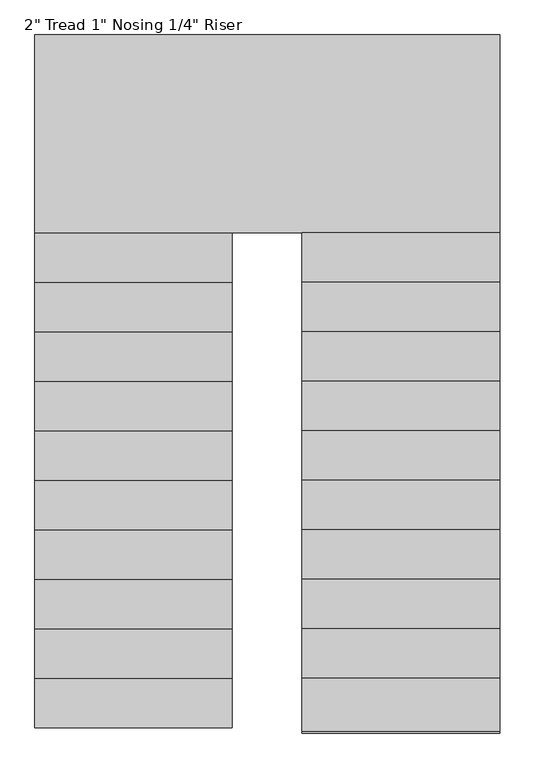
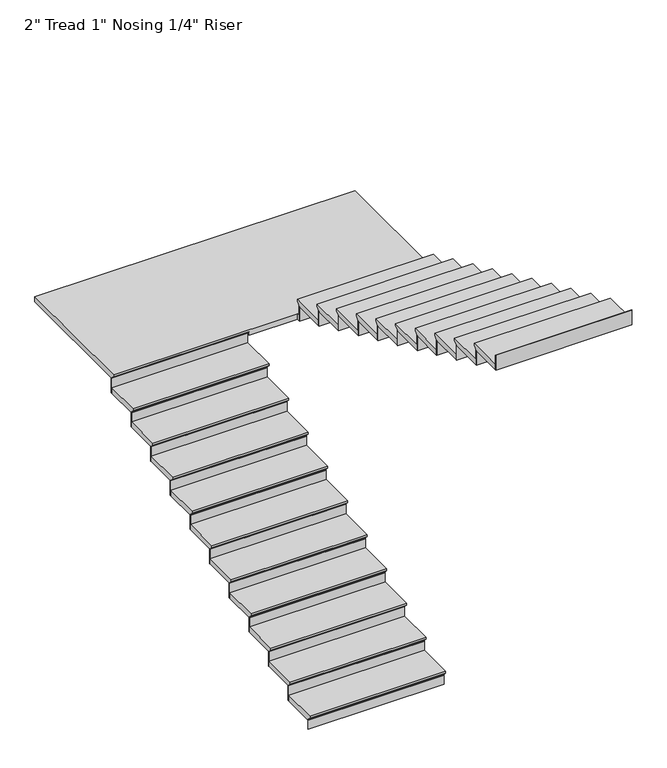
"""IFC4 building model written with IfcOpenShell, lengths in millimetres: stair flight geometry."""

from ifc_helpers import new_model, si_unit, origin, place, context, project, spatial, faceted_brep, source, transform, mapped, element, save


def stair_flight_f18b4829(model_context):
    return source(origin(), model_context, "Body", "Brep", [
        faceted_brep([(-629.5987998, 3364.6067329, 22522.2954545), (-629.5987998, 3364.6067329, 22541.3454545), (-1845.5417538, 3364.6067329, 22541.3454545), (-1845.5417538, 3364.6067329, 22522.2954545), (-629.5987998, 3390.0067329, 22496.8954545), (-1845.5417538, 3390.0067329, 22496.8954545), (-629.5987998, 3694.8067329, 22541.3454545), (-1845.5417538, 3694.8067329, 22541.3454545), (-1845.5417538, 3390.0067329, 22490.5454545), (-1845.5417538, 3694.8067329, 22490.5454545), (-629.5987998, 3694.8067329, 22490.5454545), (-629.5987998, 3390.0067329, 22490.5454545)], [[[0, 1, 2, 3]], [[4, 0, 3, 5]], [[2, 1, 6, 7]], [[8, 9, 10, 11]], [[2, 7, 9, 8, 5, 3]], [[8, 11, 4, 5]], [[6, 1, 0, 4, 11, 10]], [[7, 6, 10, 9]]]),
        faceted_brep([(-629.5987998, 3390.0067329, 22490.5454545), (-629.5987998, 3390.0067329, 22402.8), (-629.5987998, 3396.3567329, 22402.8), (-629.5987998, 3396.3567329, 22490.5454545), (-1845.5417538, 3390.0067329, 22490.5454545), (-1845.5417538, 3396.3567329, 22490.5454545), (-1845.5417538, 3396.3567329, 22402.8), (-1845.5417538, 3390.0067329, 22402.8)], [[[0, 1, 2, 3]], [[4, 5, 6, 7]], [[1, 0, 4, 7]], [[2, 1, 7, 6]], [[3, 2, 6, 5]], [[0, 3, 5, 4]]]),
        faceted_brep([(-629.5987998, 3694.8067329, 22629.0909091), (-629.5987998, 3694.8067329, 22490.5454545), (-629.5987998, 3701.1567329, 22490.5454545), (-629.5987998, 3701.1567329, 22629.0909091), (-1845.5417538, 3694.8067329, 22629.0909091), (-1845.5417538, 3701.1567329, 22629.0909091), (-1845.5417538, 3701.1567329, 22490.5454545), (-1845.5417538, 3694.8067329, 22490.5454545)], [[[0, 1, 2, 3]], [[4, 5, 6, 7]], [[1, 0, 4, 7]], [[2, 1, 7, 6]], [[3, 2, 6, 5]], [[0, 3, 5, 4]]]),
        faceted_brep([(-1845.5417538, 3669.4067329, 22679.8909091), (-629.5987998, 3669.4067329, 22679.8909091), (-629.5987998, 3999.6067329, 22679.8909091), (-1845.5417538, 3999.6067329, 22679.8909091), (-1845.5417538, 3694.8067329, 22629.0909091), (-1845.5417538, 3999.6067329, 22629.0909091), (-629.5987998, 3999.6067329, 22629.0909091), (-629.5987998, 3694.8067329, 22629.0909091), (-1845.5417538, 3694.8067329, 22635.4409091), (-1845.5417538, 3669.4067329, 22660.8409091), (-629.5987998, 3694.8067329, 22635.4409091), (-629.5987998, 3669.4067329, 22660.8409091)], [[[0, 1, 2, 3]], [[4, 5, 6, 7]], [[0, 3, 5, 4, 8, 9]], [[4, 7, 10, 8]], [[2, 1, 11, 10, 7, 6]], [[3, 2, 6, 5]], [[11, 1, 0, 9]], [[10, 11, 9, 8]]]),
        faceted_brep([(-629.5987998, 3999.6067329, 22767.6363636), (-629.5987998, 3999.6067329, 22629.0909091), (-629.5987998, 4005.9567329, 22629.0909091), (-629.5987998, 4005.9567329, 22767.6363636), (-1845.5417538, 3999.6067329, 22767.6363636), (-1845.5417538, 4005.9567329, 22767.6363636), (-1845.5417538, 4005.9567329, 22629.0909091), (-1845.5417538, 3999.6067329, 22629.0909091)], [[[0, 1, 2, 3]], [[4, 5, 6, 7]], [[1, 0, 4, 7]], [[2, 1, 7, 6]], [[3, 2, 6, 5]], [[0, 3, 5, 4]]]),
        faceted_brep([(-1845.5417538, 3974.2067329, 22818.4363636), (-629.5987998, 3974.2067329, 22818.4363636), (-629.5987998, 4304.4067329, 22818.4363636), (-1845.5417538, 4304.4067329, 22818.4363636), (-1845.5417538, 3999.6067329, 22767.6363636), (-1845.5417538, 4304.4067329, 22767.6363636), (-629.5987998, 4304.4067329, 22767.6363636), (-629.5987998, 3999.6067329, 22767.6363636), (-1845.5417538, 3999.6067329, 22773.9863636), (-1845.5417538, 3974.2067329, 22799.3863636), (-629.5987998, 3999.6067329, 22773.9863636), (-629.5987998, 3974.2067329, 22799.3863636)], [[[0, 1, 2, 3]], [[4, 5, 6, 7]], [[0, 3, 5, 4, 8, 9]], [[4, 7, 10, 8]], [[2, 1, 11, 10, 7, 6]], [[3, 2, 6, 5]], [[11, 1, 0, 9]], [[10, 11, 9, 8]]]),
        faceted_brep([(-629.5987998, 4304.4067329, 22906.1818182), (-629.5987998, 4304.4067329, 22767.6363636), (-629.5987998, 4310.7567329, 22767.6363636), (-629.5987998, 4310.7567329, 22906.1818182), (-1845.5417538, 4304.4067329, 22906.1818182), (-1845.5417538, 4310.7567329, 22906.1818182), (-1845.5417538, 4310.7567329, 22767.6363636), (-1845.5417538, 4304.4067329, 22767.6363636)], [[[0, 1, 2, 3]], [[4, 5, 6, 7]], [[1, 0, 4, 7]], [[2, 1, 7, 6]], [[3, 2, 6, 5]], [[0, 3, 5, 4]]]),
        faceted_brep([(-1845.5417538, 4279.0067329, 22956.9818182), (-629.5987998, 4279.0067329, 22956.9818182), (-629.5987998, 4609.2067329, 22956.9818182), (-1845.5417538, 4609.2067329, 22956.9818182), (-1845.5417538, 4304.4067329, 22906.1818182), (-1845.5417538, 4609.2067329, 22906.1818182), (-629.5987998, 4609.2067329, 22906.1818182), (-629.5987998, 4304.4067329, 22906.1818182), (-1845.5417538, 4304.4067329, 22912.5318182), (-1845.5417538, 4279.0067329, 22937.9318182), (-629.5987998, 4304.4067329, 22912.5318182), (-629.5987998, 4279.0067329, 22937.9318182)], [[[0, 1, 2, 3]], [[4, 5, 6, 7]], [[0, 3, 5, 4, 8, 9]], [[4, 7, 10, 8]], [[2, 1, 11, 10, 7, 6]], [[3, 2, 6, 5]], [[11, 1, 0, 9]], [[10, 11, 9, 8]]]),
        faceted_brep([(-629.5987998, 4609.2067329, 23044.7272727), (-629.5987998, 4609.2067329, 22906.1818182), (-629.5987998, 4615.5567329, 22906.1818182), (-629.5987998, 4615.5567329, 23044.7272727), (-1845.5417538, 4609.2067329, 23044.7272727), (-1845.5417538, 4615.5567329, 23044.7272727), (-1845.5417538, 4615.5567329, 22906.1818182), (-1845.5417538, 4609.2067329, 22906.1818182)], [[[0, 1, 2, 3]], [[4, 5, 6, 7]], [[1, 0, 4, 7]], [[2, 1, 7, 6]], [[3, 2, 6, 5]], [[0, 3, 5, 4]]]),
        faceted_brep([(-1845.5417538, 4583.8067329, 23095.5272727), (-629.5987998, 4583.8067329, 23095.5272727), (-629.5987998, 4914.0067329, 23095.5272727), (-1845.5417538, 4914.0067329, 23095.5272727), (-1845.5417538, 4609.2067329, 23044.7272727), (-1845.5417538, 4914.0067329, 23044.7272727), (-629.5987998, 4914.0067329, 23044.7272727), (-629.5987998, 4609.2067329, 23044.7272727), (-1845.5417538, 4609.2067329, 23051.0772727), (-1845.5417538, 4583.8067329, 23076.4772727), (-629.5987998, 4609.2067329, 23051.0772727), (-629.5987998, 4583.8067329, 23076.4772727)], [[[0, 1, 2, 3]], [[4, 5, 6, 7]], [[0, 3, 5, 4, 8, 9]], [[4, 7, 10, 8]], [[2, 1, 11, 10, 7, 6]], [[3, 2, 6, 5]], [[11, 1, 0, 9]], [[10, 11, 9, 8]]]),
        faceted_brep([(-629.5987998, 4914.0067329, 23183.2727273), (-629.5987998, 4914.0067329, 23044.7272727), (-629.5987998, 4920.3567329, 23044.7272727), (-629.5987998, 4920.3567329, 23183.2727273), (-1845.5417538, 4914.0067329, 23183.2727273), (-1845.5417538, 4920.3567329, 23183.2727273), (-1845.5417538, 4920.3567329, 23044.7272727), (-1845.5417538, 4914.0067329, 23044.7272727)], [[[0, 1, 2, 3]], [[4, 5, 6, 7]], [[1, 0, 4, 7]], [[2, 1, 7, 6]], [[3, 2, 6, 5]], [[0, 3, 5, 4]]]),
        faceted_brep([(-1845.5417538, 4888.6067329, 23234.0727273), (-629.5987998, 4888.6067329, 23234.0727273), (-629.5987998, 5218.8067329, 23234.0727273), (-1845.5417538, 5218.8067329, 23234.0727273), (-1845.5417538, 4914.0067329, 23183.2727273), (-1845.5417538, 5218.8067329, 23183.2727273), (-629.5987998, 5218.8067329, 23183.2727273), (-629.5987998, 4914.0067329, 23183.2727273), (-1845.5417538, 4914.0067329, 23189.6227273), (-1845.5417538, 4888.6067329, 23215.0227273), (-629.5987998, 4914.0067329, 23189.6227273), (-629.5987998, 4888.6067329, 23215.0227273)], [[[0, 1, 2, 3]], [[4, 5, 6, 7]], [[0, 3, 5, 4, 8, 9]], [[4, 7, 10, 8]], [[2, 1, 11, 10, 7, 6]], [[3, 2, 6, 5]], [[11, 1, 0, 9]], [[10, 11, 9, 8]]]),
        faceted_brep([(-629.5987998, 5218.8067329, 23321.8181818), (-629.5987998, 5218.8067329, 23183.2727273), (-629.5987998, 5225.1567329, 23183.2727273), (-629.5987998, 5225.1567329, 23321.8181818), (-1845.5417538, 5218.8067329, 23321.8181818), (-1845.5417538, 5225.1567329, 23321.8181818), (-1845.5417538, 5225.1567329, 23183.2727273), (-1845.5417538, 5218.8067329, 23183.2727273)], [[[0, 1, 2, 3]], [[4, 5, 6, 7]], [[1, 0, 4, 7]], [[2, 1, 7, 6]], [[3, 2, 6, 5]], [[0, 3, 5, 4]]]),
        faceted_brep([(-1845.5417538, 5193.4067329, 23372.6181818), (-629.5987998, 5193.4067329, 23372.6181818), (-629.5987998, 5523.6067329, 23372.6181818), (-1845.5417538, 5523.6067329, 23372.6181818), (-1845.5417538, 5218.8067329, 23321.8181818), (-1845.5417538, 5523.6067329, 23321.8181818), (-629.5987998, 5523.6067329, 23321.8181818), (-629.5987998, 5218.8067329, 23321.8181818), (-1845.5417538, 5218.8067329, 23328.1681818), (-1845.5417538, 5193.4067329, 23353.5681818), (-629.5987998, 5218.8067329, 23328.1681818), (-629.5987998, 5193.4067329, 23353.5681818)], [[[0, 1, 2, 3]], [[4, 5, 6, 7]], [[0, 3, 5, 4, 8, 9]], [[4, 7, 10, 8]], [[2, 1, 11, 10, 7, 6]], [[3, 2, 6, 5]], [[11, 1, 0, 9]], [[10, 11, 9, 8]]]),
        faceted_brep([(-629.5987998, 5523.6067329, 23460.3636364), (-629.5987998, 5523.6067329, 23321.8181818), (-629.5987998, 5529.9567329, 23321.8181818), (-629.5987998, 5529.9567329, 23460.3636364), (-1845.5417538, 5523.6067329, 23460.3636364), (-1845.5417538, 5529.9567329, 23460.3636364), (-1845.5417538, 5529.9567329, 23321.8181818), (-1845.5417538, 5523.6067329, 23321.8181818)], [[[0, 1, 2, 3]], [[4, 5, 6, 7]], [[1, 0, 4, 7]], [[2, 1, 7, 6]], [[3, 2, 6, 5]], [[0, 3, 5, 4]]]),
        faceted_brep([(-1845.5417538, 5498.2067329, 23511.1636364), (-629.5987998, 5498.2067329, 23511.1636364), (-629.5987998, 5828.4067329, 23511.1636364), (-1845.5417538, 5828.4067329, 23511.1636364), (-1845.5417538, 5523.6067329, 23460.3636364), (-1845.5417538, 5828.4067329, 23460.3636364), (-629.5987998, 5828.4067329, 23460.3636364), (-629.5987998, 5523.6067329, 23460.3636364), (-1845.5417538, 5523.6067329, 23466.7136364), (-1845.5417538, 5498.2067329, 23492.1136364), (-629.5987998, 5523.6067329, 23466.7136364), (-629.5987998, 5498.2067329, 23492.1136364)], [[[0, 1, 2, 3]], [[4, 5, 6, 7]], [[0, 3, 5, 4, 8, 9]], [[4, 7, 10, 8]], [[2, 1, 11, 10, 7, 6]], [[3, 2, 6, 5]], [[11, 1, 0, 9]], [[10, 11, 9, 8]]]),
        faceted_brep([(-629.5987998, 5828.4067329, 23598.9090909), (-629.5987998, 5828.4067329, 23460.3636364), (-629.5987998, 5834.7567329, 23460.3636364), (-629.5987998, 5834.7567329, 23598.9090909), (-1845.5417538, 5828.4067329, 23598.9090909), (-1845.5417538, 5834.7567329, 23598.9090909), (-1845.5417538, 5834.7567329, 23460.3636364), (-1845.5417538, 5828.4067329, 23460.3636364)], [[[0, 1, 2, 3]], [[4, 5, 6, 7]], [[1, 0, 4, 7]], [[2, 1, 7, 6]], [[3, 2, 6, 5]], [[0, 3, 5, 4]]]),
        faceted_brep([(-1845.5417538, 5803.0067329, 23649.7090909), (-629.5987998, 5803.0067329, 23649.7090909), (-629.5987998, 6133.2067329, 23649.7090909), (-1845.5417538, 6133.2067329, 23649.7090909), (-1845.5417538, 5828.4067329, 23598.9090909), (-1845.5417538, 6133.2067329, 23598.9090909), (-629.5987998, 6133.2067329, 23598.9090909), (-629.5987998, 5828.4067329, 23598.9090909), (-1845.5417538, 5828.4067329, 23605.2590909), (-1845.5417538, 5803.0067329, 23630.6590909), (-629.5987998, 5828.4067329, 23605.2590909), (-629.5987998, 5803.0067329, 23630.6590909)], [[[0, 1, 2, 3]], [[4, 5, 6, 7]], [[0, 3, 5, 4, 8, 9]], [[4, 7, 10, 8]], [[2, 1, 11, 10, 7, 6]], [[3, 2, 6, 5]], [[11, 1, 0, 9]], [[10, 11, 9, 8]]]),
        faceted_brep([(-629.5987998, 6133.2067329, 23737.4545455), (-629.5987998, 6133.2067329, 23598.9090909), (-629.5987998, 6139.5567329, 23598.9090909), (-629.5987998, 6139.5567329, 23737.4545455), (-1845.5417538, 6133.2067329, 23737.4545455), (-1845.5417538, 6139.5567329, 23737.4545455), (-1845.5417538, 6139.5567329, 23598.9090909), (-1845.5417538, 6133.2067329, 23598.9090909)], [[[0, 1, 2, 3]], [[4, 5, 6, 7]], [[1, 0, 4, 7]], [[2, 1, 7, 6]], [[3, 2, 6, 5]], [[0, 3, 5, 4]]]),
        faceted_brep([(-1845.5417538, 6107.8067329, 23788.2545455), (-629.5987998, 6107.8067329, 23788.2545455), (-629.5987998, 6438.0067329, 23788.2545455), (-1845.5417538, 6438.0067329, 23788.2545455), (-1845.5417538, 6133.2067329, 23737.4545455), (-1845.5417538, 6438.0067329, 23737.4545455), (-629.5987998, 6438.0067329, 23737.4545455), (-629.5987998, 6133.2067329, 23737.4545455), (-1845.5417538, 6133.2067329, 23743.8045455), (-1845.5417538, 6107.8067329, 23769.2045455), (-629.5987998, 6133.2067329, 23743.8045455), (-629.5987998, 6107.8067329, 23769.2045455)], [[[0, 1, 2, 3]], [[4, 5, 6, 7]], [[0, 3, 5, 4, 8, 9]], [[4, 7, 10, 8]], [[2, 1, 11, 10, 7, 6]], [[3, 2, 6, 5]], [[11, 1, 0, 9]], [[10, 11, 9, 8]]]),
        faceted_brep([(-629.5987998, 6438.0067329, 23876.0), (-629.5987998, 6438.0067329, 23737.4545455), (-629.5987998, 6444.3567329, 23737.4545455), (-629.5987998, 6444.3567329, 23876.0), (-1845.5417538, 6438.0067329, 23876.0), (-1845.5417538, 6444.3567329, 23876.0), (-1845.5417538, 6444.3567329, 23737.4545455), (-1845.5417538, 6438.0067329, 23737.4545455)], [[[0, 1, 2, 3]], [[4, 5, 6, 7]], [[1, 0, 4, 7]], [[2, 1, 7, 6]], [[3, 2, 6, 5]], [[0, 3, 5, 4]]]),
        faceted_brep([(1021.4012085, 6387.2067329, 23926.8), (1021.4012085, 7631.8067329, 23926.8), (-1845.5417538, 7631.8067329, 23926.8), (-1845.5417538, 6412.6067329, 23926.8), (-197.7987915, 6412.6067329, 23926.8), (-197.7987915, 6387.2067329, 23926.8), (1021.4012085, 7631.8067329, 23876.0), (1021.4012085, 6387.2067329, 23876.0), (-197.7987915, 6387.2067329, 23876.0), (-197.7987915, 6412.6067329, 23876.0), (-629.5987998, 6412.6067329, 23876.0), (-629.5987998, 6438.0067329, 23876.0), (-1845.5417538, 6438.0067329, 23876.0), (-1845.5417538, 7631.8067329, 23876.0), (-629.5987998, 6438.0067329, 23882.35), (-1845.5417538, 6438.0067329, 23882.35), (-1845.5417538, 6412.6067329, 23907.75), (-629.5987998, 6412.6067329, 23907.75)], [[[0, 1, 2, 3, 4, 5]], [[6, 7, 8, 9, 10, 11, 12, 13]], [[1, 0, 7, 6]], [[2, 1, 6, 13]], [[12, 11, 14, 15]], [[4, 3, 16, 17, 10, 9]], [[5, 4, 9, 8]], [[0, 5, 8, 7]], [[16, 15, 14, 17]], [[3, 2, 13, 12, 15, 16]], [[11, 10, 17, 14]]]),
        faceted_brep([(-197.7987915, 6387.2067329, 24014.5454545), (-197.7987915, 6387.2067329, 23876.0), (-197.7987915, 6380.8567329, 23876.0), (-197.7987915, 6380.8567329, 24014.5454545), (1021.4012085, 6387.2067329, 24014.5454545), (1021.4012085, 6380.8567329, 24014.5454545), (1021.4012085, 6380.8567329, 23876.0), (1021.4012085, 6387.2067329, 23876.0)], [[[0, 1, 2, 3]], [[4, 5, 6, 7]], [[1, 0, 4, 7]], [[2, 1, 7, 6]], [[3, 2, 6, 5]], [[0, 3, 5, 4]]]),
        faceted_brep([(1021.4012085, 6412.6067329, 24065.3454545), (-197.7987915, 6412.6067329, 24065.3454545), (-197.7987915, 6082.4067329, 24065.3454545), (1021.4012085, 6082.4067329, 24065.3454545), (1021.4012085, 6387.2067329, 24014.5454545), (1021.4012085, 6082.4067329, 24014.5454545), (-197.7987915, 6082.4067329, 24014.5454545), (-197.7987915, 6387.2067329, 24014.5454545), (1021.4012085, 6387.2067329, 24020.8954545), (1021.4012085, 6412.6067329, 24046.2954545), (-197.7987915, 6387.2067329, 24020.8954545), (-197.7987915, 6412.6067329, 24046.2954545)], [[[0, 1, 2, 3]], [[4, 5, 6, 7]], [[0, 3, 5, 4, 8, 9]], [[4, 7, 10, 8]], [[2, 1, 11, 10, 7, 6]], [[3, 2, 6, 5]], [[11, 1, 0, 9]], [[10, 11, 9, 8]]]),
        faceted_brep([(-197.7987915, 6082.4067329, 24153.0909091), (-197.7987915, 6082.4067329, 24014.5454545), (-197.7987915, 6076.0567329, 24014.5454545), (-197.7987915, 6076.0567329, 24153.0909091), (1021.4012085, 6082.4067329, 24153.0909091), (1021.4012085, 6076.0567329, 24153.0909091), (1021.4012085, 6076.0567329, 24014.5454545), (1021.4012085, 6082.4067329, 24014.5454545)], [[[0, 1, 2, 3]], [[4, 5, 6, 7]], [[1, 0, 4, 7]], [[2, 1, 7, 6]], [[3, 2, 6, 5]], [[0, 3, 5, 4]]]),
        faceted_brep([(1021.4012085, 6107.8067329, 24203.8909091), (-197.7987915, 6107.8067329, 24203.8909091), (-197.7987915, 5777.6067329, 24203.8909091), (1021.4012085, 5777.6067329, 24203.8909091), (1021.4012085, 6082.4067329, 24153.0909091), (1021.4012085, 5777.6067329, 24153.0909091), (-197.7987915, 5777.6067329, 24153.0909091), (-197.7987915, 6082.4067329, 24153.0909091), (1021.4012085, 6082.4067329, 24159.4409091), (1021.4012085, 6107.8067329, 24184.8409091), (-197.7987915, 6082.4067329, 24159.4409091), (-197.7987915, 6107.8067329, 24184.8409091)], [[[0, 1, 2, 3]], [[4, 5, 6, 7]], [[0, 3, 5, 4, 8, 9]], [[4, 7, 10, 8]], [[2, 1, 11, 10, 7, 6]], [[3, 2, 6, 5]], [[11, 1, 0, 9]], [[10, 11, 9, 8]]]),
        faceted_brep([(-197.7987915, 5777.6067329, 24291.6363636), (-197.7987915, 5777.6067329, 24153.0909091), (-197.7987915, 5771.2567329, 24153.0909091), (-197.7987915, 5771.2567329, 24291.6363636), (1021.4012085, 5777.6067329, 24291.6363636), (1021.4012085, 5771.2567329, 24291.6363636), (1021.4012085, 5771.2567329, 24153.0909091), (1021.4012085, 5777.6067329, 24153.0909091)], [[[0, 1, 2, 3]], [[4, 5, 6, 7]], [[1, 0, 4, 7]], [[2, 1, 7, 6]], [[3, 2, 6, 5]], [[0, 3, 5, 4]]]),
        faceted_brep([(1021.4012085, 5803.0067329, 24342.4363636), (-197.7987915, 5803.0067329, 24342.4363636), (-197.7987915, 5472.8067329, 24342.4363636), (1021.4012085, 5472.8067329, 24342.4363636), (1021.4012085, 5777.6067329, 24291.6363636), (1021.4012085, 5472.8067329, 24291.6363636), (-197.7987915, 5472.8067329, 24291.6363636), (-197.7987915, 5777.6067329, 24291.6363636), (1021.4012085, 5777.6067329, 24297.9863636), (1021.4012085, 5803.0067329, 24323.3863636), (-197.7987915, 5777.6067329, 24297.9863636), (-197.7987915, 5803.0067329, 24323.3863636)], [[[0, 1, 2, 3]], [[4, 5, 6, 7]], [[0, 3, 5, 4, 8, 9]], [[4, 7, 10, 8]], [[2, 1, 11, 10, 7, 6]], [[3, 2, 6, 5]], [[11, 1, 0, 9]], [[10, 11, 9, 8]]]),
        faceted_brep([(-197.7987915, 5472.8067329, 24430.1818182), (-197.7987915, 5472.8067329, 24291.6363636), (-197.7987915, 5466.4567329, 24291.6363636), (-197.7987915, 5466.4567329, 24430.1818182), (1021.4012085, 5472.8067329, 24430.1818182), (1021.4012085, 5466.4567329, 24430.1818182), (1021.4012085, 5466.4567329, 24291.6363636), (1021.4012085, 5472.8067329, 24291.6363636)], [[[0, 1, 2, 3]], [[4, 5, 6, 7]], [[1, 0, 4, 7]], [[2, 1, 7, 6]], [[3, 2, 6, 5]], [[0, 3, 5, 4]]]),
        faceted_brep([(1021.4012085, 5498.2067329, 24480.9818182), (-197.7987915, 5498.2067329, 24480.9818182), (-197.7987915, 5168.0067329, 24480.9818182), (1021.4012085, 5168.0067329, 24480.9818182), (1021.4012085, 5472.8067329, 24430.1818182), (1021.4012085, 5168.0067329, 24430.1818182), (-197.7987915, 5168.0067329, 24430.1818182), (-197.7987915, 5472.8067329, 24430.1818182), (1021.4012085, 5472.8067329, 24436.5318182), (1021.4012085, 5498.2067329, 24461.9318182), (-197.7987915, 5472.8067329, 24436.5318182), (-197.7987915, 5498.2067329, 24461.9318182)], [[[0, 1, 2, 3]], [[4, 5, 6, 7]], [[0, 3, 5, 4, 8, 9]], [[4, 7, 10, 8]], [[2, 1, 11, 10, 7, 6]], [[3, 2, 6, 5]], [[11, 1, 0, 9]], [[10, 11, 9, 8]]]),
        faceted_brep([(-197.7987915, 5168.0067329, 24568.7272727), (-197.7987915, 5168.0067329, 24430.1818182), (-197.7987915, 5161.6567329, 24430.1818182), (-197.7987915, 5161.6567329, 24568.7272727), (1021.4012085, 5168.0067329, 24568.7272727), (1021.4012085, 5161.6567329, 24568.7272727), (1021.4012085, 5161.6567329, 24430.1818182), (1021.4012085, 5168.0067329, 24430.1818182)], [[[0, 1, 2, 3]], [[4, 5, 6, 7]], [[1, 0, 4, 7]], [[2, 1, 7, 6]], [[3, 2, 6, 5]], [[0, 3, 5, 4]]]),
        faceted_brep([(1021.4012085, 5193.4067329, 24619.5272727), (-197.7987915, 5193.4067329, 24619.5272727), (-197.7987915, 4863.2067329, 24619.5272727), (1021.4012085, 4863.2067329, 24619.5272727), (1021.4012085, 5168.0067329, 24568.7272727), (1021.4012085, 4863.2067329, 24568.7272727), (-197.7987915, 4863.2067329, 24568.7272727), (-197.7987915, 5168.0067329, 24568.7272727), (1021.4012085, 5168.0067329, 24575.0772727), (1021.4012085, 5193.4067329, 24600.4772727), (-197.7987915, 5168.0067329, 24575.0772727), (-197.7987915, 5193.4067329, 24600.4772727)], [[[0, 1, 2, 3]], [[4, 5, 6, 7]], [[0, 3, 5, 4, 8, 9]], [[4, 7, 10, 8]], [[2, 1, 11, 10, 7, 6]], [[3, 2, 6, 5]], [[11, 1, 0, 9]], [[10, 11, 9, 8]]]),
        faceted_brep([(-197.7987915, 4863.2067329, 24707.2727273), (-197.7987915, 4863.2067329, 24568.7272727), (-197.7987915, 4856.8567329, 24568.7272727), (-197.7987915, 4856.8567329, 24707.2727273), (1021.4012085, 4863.2067329, 24707.2727273), (1021.4012085, 4856.8567329, 24707.2727273), (1021.4012085, 4856.8567329, 24568.7272727), (1021.4012085, 4863.2067329, 24568.7272727)], [[[0, 1, 2, 3]], [[4, 5, 6, 7]], [[1, 0, 4, 7]], [[2, 1, 7, 6]], [[3, 2, 6, 5]], [[0, 3, 5, 4]]]),
        faceted_brep([(1021.4012085, 4888.6067329, 24758.0727273), (-197.7987915, 4888.6067329, 24758.0727273), (-197.7987915, 4558.4067329, 24758.0727273), (1021.4012085, 4558.4067329, 24758.0727273), (1021.4012085, 4863.2067329, 24707.2727273), (1021.4012085, 4558.4067329, 24707.2727273), (-197.7987915, 4558.4067329, 24707.2727273), (-197.7987915, 4863.2067329, 24707.2727273), (1021.4012085, 4863.2067329, 24713.6227273), (1021.4012085, 4888.6067329, 24739.0227273), (-197.7987915, 4863.2067329, 24713.6227273), (-197.7987915, 4888.6067329, 24739.0227273)], [[[0, 1, 2, 3]], [[4, 5, 6, 7]], [[0, 3, 5, 4, 8, 9]], [[4, 7, 10, 8]], [[2, 1, 11, 10, 7, 6]], [[3, 2, 6, 5]], [[11, 1, 0, 9]], [[10, 11, 9, 8]]]),
        faceted_brep([(-197.7987915, 4558.4067329, 24845.8181818), (-197.7987915, 4558.4067329, 24707.2727273), (-197.7987915, 4552.0567329, 24707.2727273), (-197.7987915, 4552.0567329, 24845.8181818), (1021.4012085, 4558.4067329, 24845.8181818), (1021.4012085, 4552.0567329, 24845.8181818), (1021.4012085, 4552.0567329, 24707.2727273), (1021.4012085, 4558.4067329, 24707.2727273)], [[[0, 1, 2, 3]], [[4, 5, 6, 7]], [[1, 0, 4, 7]], [[2, 1, 7, 6]], [[3, 2, 6, 5]], [[0, 3, 5, 4]]]),
        faceted_brep([(1021.4012085, 4583.8067329, 24896.6181818), (-197.7987915, 4583.8067329, 24896.6181818), (-197.7987915, 4253.6067329, 24896.6181818), (1021.4012085, 4253.6067329, 24896.6181818), (1021.4012085, 4558.4067329, 24845.8181818), (1021.4012085, 4253.6067329, 24845.8181818), (-197.7987915, 4253.6067329, 24845.8181818), (-197.7987915, 4558.4067329, 24845.8181818), (1021.4012085, 4558.4067329, 24852.1681818), (1021.4012085, 4583.8067329, 24877.5681818), (-197.7987915, 4558.4067329, 24852.1681818), (-197.7987915, 4583.8067329, 24877.5681818)], [[[0, 1, 2, 3]], [[4, 5, 6, 7]], [[0, 3, 5, 4, 8, 9]], [[4, 7, 10, 8]], [[2, 1, 11, 10, 7, 6]], [[3, 2, 6, 5]], [[11, 1, 0, 9]], [[10, 11, 9, 8]]]),
        faceted_brep([(-197.7987915, 4253.6067329, 24984.3636364), (-197.7987915, 4253.6067329, 24845.8181818), (-197.7987915, 4247.2567329, 24845.8181818), (-197.7987915, 4247.2567329, 24984.3636364), (1021.4012085, 4253.6067329, 24984.3636364), (1021.4012085, 4247.2567329, 24984.3636364), (1021.4012085, 4247.2567329, 24845.8181818), (1021.4012085, 4253.6067329, 24845.8181818)], [[[0, 1, 2, 3]], [[4, 5, 6, 7]], [[1, 0, 4, 7]], [[2, 1, 7, 6]], [[3, 2, 6, 5]], [[0, 3, 5, 4]]]),
        faceted_brep([(1021.4012085, 4279.0067329, 25035.1636364), (-197.7987915, 4279.0067329, 25035.1636364), (-197.7987915, 3948.8067329, 25035.1636364), (1021.4012085, 3948.8067329, 25035.1636364), (1021.4012085, 4253.6067329, 24984.3636364), (1021.4012085, 3948.8067329, 24984.3636364), (-197.7987915, 3948.8067329, 24984.3636364), (-197.7987915, 4253.6067329, 24984.3636364), (1021.4012085, 4253.6067329, 24990.7136364), (1021.4012085, 4279.0067329, 25016.1136364), (-197.7987915, 4253.6067329, 24990.7136364), (-197.7987915, 4279.0067329, 25016.1136364)], [[[0, 1, 2, 3]], [[4, 5, 6, 7]], [[0, 3, 5, 4, 8, 9]], [[4, 7, 10, 8]], [[2, 1, 11, 10, 7, 6]], [[3, 2, 6, 5]], [[11, 1, 0, 9]], [[10, 11, 9, 8]]]),
        faceted_brep([(-197.7987915, 3948.8067329, 25122.9090909), (-197.7987915, 3948.8067329, 24984.3636364), (-197.7987915, 3942.4567329, 24984.3636364), (-197.7987915, 3942.4567329, 25122.9090909), (1021.4012085, 3948.8067329, 25122.9090909), (1021.4012085, 3942.4567329, 25122.9090909), (1021.4012085, 3942.4567329, 24984.3636364), (1021.4012085, 3948.8067329, 24984.3636364)], [[[0, 1, 2, 3]], [[4, 5, 6, 7]], [[1, 0, 4, 7]], [[2, 1, 7, 6]], [[3, 2, 6, 5]], [[0, 3, 5, 4]]]),
        faceted_brep([(1021.4012085, 3974.2067329, 25173.7090909), (-197.7987915, 3974.2067329, 25173.7090909), (-197.7987915, 3644.0067329, 25173.7090909), (1021.4012085, 3644.0067329, 25173.7090909), (1021.4012085, 3948.8067329, 25122.9090909), (1021.4012085, 3644.0067329, 25122.9090909), (-197.7987915, 3644.0067329, 25122.9090909), (-197.7987915, 3948.8067329, 25122.9090909), (1021.4012085, 3948.8067329, 25129.2590909), (1021.4012085, 3974.2067329, 25154.6590909), (-197.7987915, 3948.8067329, 25129.2590909), (-197.7987915, 3974.2067329, 25154.6590909)], [[[0, 1, 2, 3]], [[4, 5, 6, 7]], [[0, 3, 5, 4, 8, 9]], [[4, 7, 10, 8]], [[2, 1, 11, 10, 7, 6]], [[3, 2, 6, 5]], [[11, 1, 0, 9]], [[10, 11, 9, 8]]]),
        faceted_brep([(-197.7987915, 3644.0067329, 25261.4545455), (-197.7987915, 3644.0067329, 25122.9090909), (-197.7987915, 3637.6567329, 25122.9090909), (-197.7987915, 3637.6567329, 25261.4545455), (1021.4012085, 3644.0067329, 25261.4545455), (1021.4012085, 3637.6567329, 25261.4545455), (1021.4012085, 3637.6567329, 25122.9090909), (1021.4012085, 3644.0067329, 25122.9090909)], [[[0, 1, 2, 3]], [[4, 5, 6, 7]], [[1, 0, 4, 7]], [[2, 1, 7, 6]], [[3, 2, 6, 5]], [[0, 3, 5, 4]]]),
        faceted_brep([(-197.7987915, 3339.2067329, 25400.0), (-197.7987915, 3339.2067329, 25261.4545455), (-197.7987915, 3332.8567329, 25261.4545455), (-197.7987915, 3332.8567329, 25400.0), (1021.4012085, 3339.2067329, 25400.0), (1021.4012085, 3332.8567329, 25400.0), (1021.4012085, 3332.8567329, 25261.4545455), (1021.4012085, 3339.2067329, 25261.4545455)], [[[0, 1, 2, 3]], [[4, 5, 6, 7]], [[1, 0, 4, 7]], [[2, 1, 7, 6]], [[3, 2, 6, 5]], [[0, 3, 5, 4]]]),
        faceted_brep([(1021.4012085, 3669.4067329, 25312.2545455), (-197.7987915, 3669.4067329, 25312.2545455), (-197.7987915, 3339.2067329, 25312.2545455), (1021.4012085, 3339.2067329, 25312.2545455), (1021.4012085, 3644.0067329, 25261.4545455), (1021.4012085, 3339.2067329, 25261.4545455), (-197.7987915, 3339.2067329, 25261.4545455), (-197.7987915, 3644.0067329, 25261.4545455), (1021.4012085, 3644.0067329, 25267.8045455), (1021.4012085, 3669.4067329, 25293.2045455), (-197.7987915, 3644.0067329, 25267.8045455), (-197.7987915, 3669.4067329, 25293.2045455)], [[[0, 1, 2, 3]], [[4, 5, 6, 7]], [[0, 3, 5, 4, 8, 9]], [[4, 7, 10, 8]], [[2, 1, 11, 10, 7, 6]], [[3, 2, 6, 5]], [[11, 1, 0, 9]], [[10, 11, 9, 8]]]),
    ])


if __name__ == "__main__":
    model = new_model("IFC4")
    model_context = context("Model", 3, world=origin())
    ifc_project = project(units=[si_unit("LENGTHUNIT", "METRE", prefix="MILLI")], contexts=[model_context])
    site = spatial("IfcSite", under=ifc_project)
    building = spatial("IfcBuilding", under=site)
    placement = place(None, origin())
    stair_flight_shape = stair_flight_f18b4829(model_context)
    element("IfcStairFlight", 1, ObjectType="2\" Tread 1\" Nosing 1/4\" Riser", at=placement, inside=building, context=model_context, shape_type="MappedRepresentation", body=[
        mapped(stair_flight_shape, transform((0.0, 0.0, 0.0), x_axis=(1.0, 0.0, 0.0), y_axis=(0.0, 1.0, 0.0), z_axis=(0.0, 0.0, 1.0))),
    ])
    save(model, "model.ifc")
